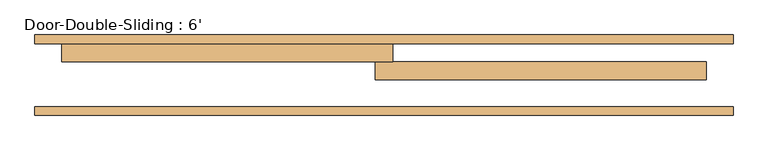
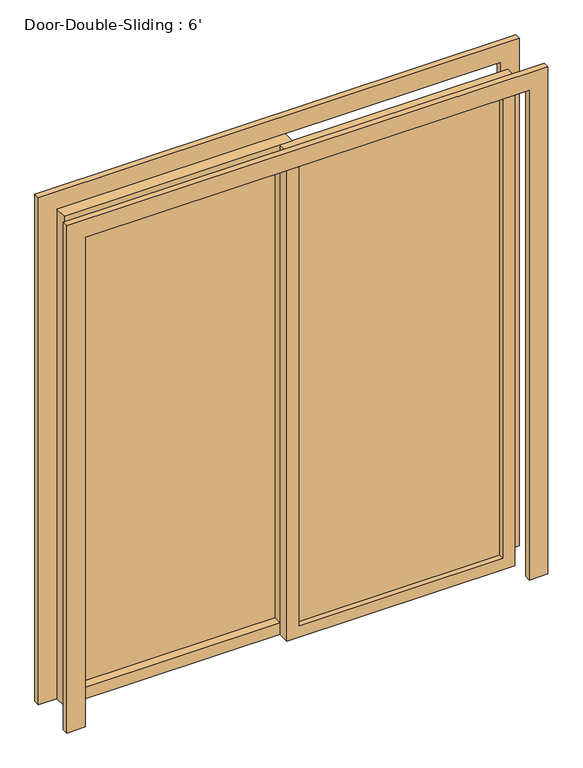
"""IFC4 building model written with IfcOpenShell, lengths in millimetres: door geometry, Door-Double-Sliding : 6'."""

from ifc_helpers import new_model, si_unit, frame, origin, place, context, project, spatial, polyline, outline, extrude, source, transform, mapped, element, save


def door_double_sliding_6_85a7ba4d(model_context):
    return source(origin(), model_context, "Body", "SweptSolid", [
        extrude(outline(polyline([(0.0, 990.6), (2209.8, 990.6), (2209.8, -990.6), (0.0, -990.6), (0.0, -914.4), (2133.6, -914.4), (2133.6, 914.4), (0.0, 914.4), (0.0, 990.6)])), frame((0.0, 215.9, 0.0), z_axis=(0.0, 1.0, 0.0), x_axis=(0.0, 0.0, 1.0)), (0.0, 0.0, 1.0), 25.4),
        extrude(outline(polyline([(0.0, -990.6), (0.0, -914.4), (2133.6, -914.4), (2133.6, 914.4), (0.0, 914.4), (0.0, 990.6), (2209.8, 990.6), (2209.8, -990.6), (0.0, -990.6)])), frame((0.0, 12.7, 0.0), z_axis=(0.0, 1.0, 0.0), x_axis=(0.0, 0.0, 1.0)), (0.0, 0.0, 1.0), 25.4),
        extrude(outline(polyline([(2133.6, 25.4), (2133.6, -914.4), (0.0, -914.4), (0.0, 25.4), (2133.6, 25.4)]), holes=[polyline([(2082.8, -25.4), (50.8, -25.4), (50.8, -863.6), (2082.8, -863.6), (2082.8, -25.4)])]), frame((0.0, 165.1, 0.0), z_axis=(0.0, 1.0, 0.0), x_axis=(0.0, 0.0, 1.0)), (0.0, 0.0, 1.0), 50.8),
        extrude(outline(polyline([(2133.6, -25.4), (0.0, -25.4), (0.0, 914.4), (2133.6, 914.4), (2133.6, -25.4)]), holes=[polyline([(2082.8, 25.4), (2082.8, 863.6), (50.8, 863.6), (50.8, 25.4), (2082.8, 25.4)])]), frame((0.0, 114.3, 0.0), z_axis=(0.0, 1.0, 0.0), x_axis=(0.0, 0.0, 1.0)), (0.0, 0.0, 1.0), 50.8),
        extrude(outline(polyline([(-25.4, 200.025), (-863.6, 200.025), (-863.6, 206.375), (-25.4, 206.375), (-25.4, 200.025)])), frame((0.0, 0.0, 50.8), z_axis=(0.0, 0.0, 1.0), x_axis=(1.0, 0.0, 0.0)), (0.0, 0.0, 1.0), 2032.0),
        extrude(outline(polyline([(25.4, 142.875), (863.6, 142.875), (863.6, 136.525), (25.4, 136.525), (25.4, 142.875)])), frame((0.0, 0.0, 50.8), z_axis=(0.0, 0.0, 1.0), x_axis=(1.0, 0.0, 0.0)), (0.0, 0.0, 1.0), 2032.0),
    ])


if __name__ == "__main__":
    model = new_model("IFC4")
    model_context = context("Model", 3, world=origin())
    ifc_project = project(units=[si_unit("LENGTHUNIT", "METRE", prefix="MILLI")], contexts=[model_context])
    site = spatial("IfcSite", under=ifc_project)
    building = spatial("IfcBuilding", under=site)
    placement = place(None, origin())
    door_double_sliding_6_shape = door_double_sliding_6_85a7ba4d(model_context)
    element("IfcDoor", 1, ObjectType="Door-Double-Sliding : 6'", at=placement, inside=building, context=model_context, shape_type="MappedRepresentation", body=[
        mapped(door_double_sliding_6_shape, transform((0.0, 0.0, 0.0), x_axis=(1.0, 0.0, 0.0), y_axis=(0.0, 1.0, 0.0), z_axis=(0.0, 0.0, 1.0))),
    ])
    save(model, "model.ifc")

# Revit data of these elements
# Type "Door-Double-Sliding : 6'"
#   Type Mark = "17"
#   Construction Type Id = "opn-d45"
#   Assembly Code = "C1020"
#   Analytic Construction = "Wood frame, double glass door "
#   Thickness = 0' - 2"
#   Thermal Resistance (R) = 1.8150 (h·ft²·°F)/BTU
#   Heat Transfer Coefficient (U) = 0.5510 BTU/(h·ft²·°F)
#   Height = 7' - 0"
#   Rail Width = 0' - 2"
#   Stiles = 0' - 2"
#   Trim Projection Ext = 0' - 1"
#   Trim Projection Int = 0' - 1"
#   Trim Width = 0' - 3"
#   Width = 6' - 0"
#   Define Thermal Properties by = 1
#   Glazing = Glass
#   Panel Material = Wood - Birch - Solid Stained Light Low Gloss
#   Trim Material = Paint - Sienna
#   Visual Light Transmittance = 0
#   Solar Heat Gain Coefficient = 0
#   Function = (empty or 0)
#   Wall Closure = (empty or 0)
# Element 1 (IfcDoor, "Door-Double-Sliding : 6'")
#   Materials on its faces: "Paint - Sienna", "Wood - Birch - Solid Stained Light Low Gloss", "Glass"
# Materials
#   "Glass": class "Glass", colour RGB 0 128 192, transparency 0.75, Description = "Soda Lime Glass", Cost = 0
#   "Wood - Birch - Solid Stained Light Low Gloss": class "Wood", colour RGB 210 159 95, transparency 0, Cost = 0
#   "Paint - Sienna": colour RGB 118 70 51, transparency 0, Cost = 0
